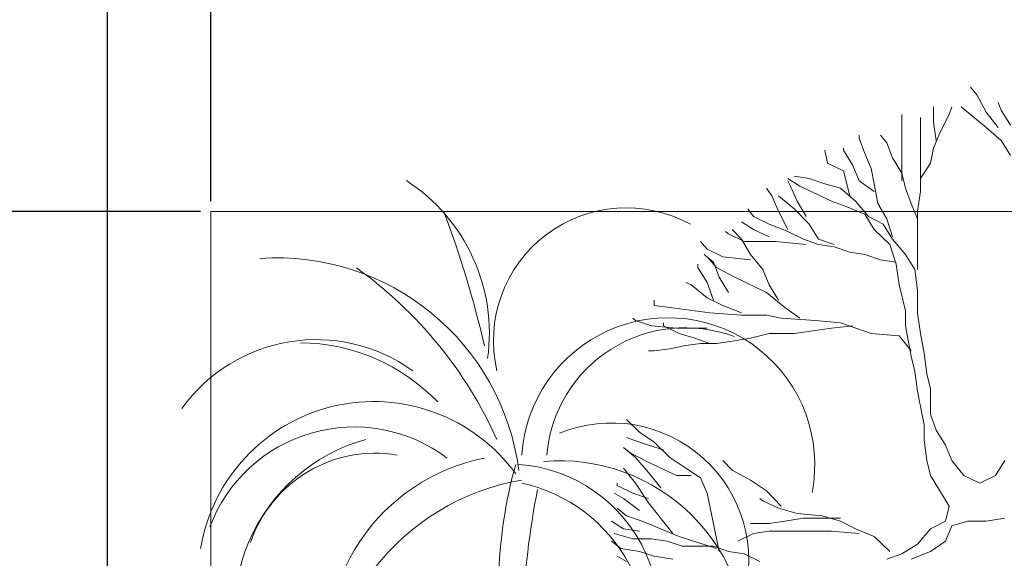
# Model space of a CAD drawing. Units: millimetres. Extents: x 595116 to 630915, y 909473 to 920225.
# Tile 51 of 134: x 629500 to 629559, y 919281 to 919314. Entities that reach past the tile are written whole.
import ezdxf

# ---------------------------------------------------------------- set-up
doc = ezdxf.new("R2010")
doc.units = ezdxf.units.MM
doc.layers.add('Dimension', color=3, linetype='Continuous', lineweight=18)
doc.layers.add('L-PLNT', color=85, linetype='Continuous', lineweight=13)
doc.styles.get("Standard").update_dxf_attribs({"font": 'arial.ttf'})
doc.dimstyles.new('ISO-25', dxfattribs={"dimtxt": 9, "dimasz": 6, "dimexe": 1.25, "dimexo": 0.625, "dimtad": 1, "dimlunit": 4, "dimtxsty": 'Standard', "dimcen": 2.5, "dimadec": 0, "dimazin": 0, "dimtfac": 1, "dimtmove": 0, "dimatfit": 3, "dimfxl": 1, "dimarcsym": 0})

# ---------------------------------------------------------------- blocks, each defined once
blk = doc.blocks.new('tree')
for centre, radius, start, end in [((629595.141, 919296.95), 5.184, 352.032, 57.0714), ((629569.835, 919289.496), 31.168, 13.149, 20.5076), ((629604.232, 919296.737), 3.791, 61.1347, 193.108), ((629594.259, 919292.132), 6.965, 7.4001, 94.0059), ((629589.446, 919288.922), 12.167, 24.2477, 54.3726), ((629605.429, 919293.205), 4.185, 348.9977, 176.315), ((629605.915, 919293.144), 3.963, 69.3845, 175.231), ((629595.377, 919292.044), 4.722, 54.2484, 144.2167), ((629594.88, 919291.171), 5.506, 43.8672, 89.4805), ((629597.025, 919289.989), 5.01, 36.0581, 170.6542), ((629596.464, 919289.874), 4.4, 52.9074, 159.3471), ((629603.809, 919290.469), 3.92, 343.886, 112.2662), ((629598.153, 919288.998), 5.103, 105.3576, 208.8973), ((629597.068, 919289.758), 3.768, 80.4816, 161.0664), ((629601.247, 919287.941), 5.545, 101.0419, 191.8692), ((629614.329, 919289.554), 13.748, 164.5925, 192.323), ((629600.849, 919288.894), 4.324, 322.5461, 85.805), ((629602.329, 919287.957), 5.355, 355.2141, 94.8217), ((629602.391, 919286.088), 6.769, 99.681, 184.5451), ((629626.813, 919287.645), 25.579, 169.0753, 185.2889), ((629600.275, 919288.191), 4.585, 338.7925, 77.6921)]:
    blk.add_arc(centre, radius, start, end)
blk = doc.blocks.new('A$C143125F4')
for p, q in [((2.1554, 4.9368), (2.1171, 4.9816)), ((2.2101, 4.8338), (2.1554, 4.9368)), ((2.2976, 4.8472), (2.2812, 4.892)), ((1.7123, 4.4306), (1.7123, 4.8203)), ((1.8983, 4.7755), (1.8983, 4.8651)), ((1.9366, 4.7128), (1.9913, 4.8203)), ((1.9913, 4.8203), (2.0077, 4.8651)), ((2.2101, 4.7442), (2.0624, 4.8651)), ((2.2812, 4.7442), (2.2101, 4.8338)), ((2.3523, 4.7576), (2.2976, 4.8472)), ((1.8217, 4.3679), (1.8217, 4.8024)), ((1.9147, 4.668), (1.8983, 4.7755)), ((1.8983, 4.6232), (1.9366, 4.7128)), ((2.2976, 4.668), (2.2101, 4.7442)), ((1.4606, 4.6814), (1.4606, 4.6994)), ((1.4935, 4.5919), (1.4606, 4.6814)), ((1.6247, 4.6546), (1.5865, 4.6994)), ((1.6576, 4.565), (1.6247, 4.6546)), ((2.3523, 4.5784), (2.2976, 4.668)), ((1.2746, 4.5336), (1.2582, 4.6098)), ((1.3676, 4.6098), (1.3676, 4.6232)), ((1.4223, 4.5202), (1.3676, 4.6098)), ((1.5317, 4.5023), (1.4935, 4.5919)), ((1.8819, 4.5336), (1.8983, 4.6232)), ((1.3676, 4.4888), (1.2746, 4.5336)), ((1.7123, 4.4754), (1.6576, 4.565)), ((1.8217, 4.444), (1.8819, 4.5336)), ((1.4059, 4.341), (1.3676, 4.4888)), ((1.4606, 4.4306), (1.4223, 4.5202)), ((1.5482, 4.4127), (1.5317, 4.5023)), ((1.7342, 4.3858), (1.7123, 4.4754)), ((1.1105, 4.3992), (1.0394, 4.444)), ((1.0558, 4.3992), (1.0394, 4.4306)), ((1.0777, 4.4575), (1.1652, 4.444)), ((1.1652, 4.444), (1.2582, 4.4127)), ((1.5482, 4.3679), (1.4606, 4.4306)), ((0.9464, 4.341), (0.9136, 4.3858)), ((1.0941, 4.3096), (1.0558, 4.3992)), ((1.2965, 4.3096), (1.1105, 4.3992)), ((1.2582, 4.4127), (1.3512, 4.3858)), ((1.3512, 4.3858), (1.4387, 4.3096)), ((1.57, 4.2962), (1.5482, 4.4127)), ((1.767, 4.2962), (1.7342, 4.3858)), ((1.8053, 4.2514), (1.8217, 4.3679)), ((0.9847, 4.2514), (0.9464, 4.341)), ((1.0777, 4.2648), (0.9847, 4.341)), ((1.1488, 4.22), (1.0941, 4.3096)), ((1.384, 4.2783), (1.2965, 4.3096)), ((1.4387, 4.3096), (1.5153, 4.22)), ((0.837, 4.22), (0.8042, 4.2648)), ((1.0394, 4.1439), (0.9847, 4.2514)), ((1.1652, 4.1752), (1.0777, 4.2648)), ((1.4935, 4.2335), (1.384, 4.2783)), ((1.6247, 4.2066), (1.57, 4.2962)), ((1.8053, 4.2066), (1.767, 4.2962)), ((1.8053, 3.9064), (1.8053, 4.2514)), ((0.837, 4.1439), (0.7659, 4.1887)), ((0.93, 4.1752), (0.837, 4.22)), ((1.5482, 4.1439), (1.4935, 4.2335)), ((1.5153, 4.22), (1.6029, 4.1752)), ((1.6576, 4.0991), (1.6247, 4.2066)), ((0.6893, 4.117), (0.6729, 4.1304)), ((0.7659, 4.0856), (0.7112, 4.1439)), ((0.93, 4.0991), (0.837, 4.1439)), ((1.0394, 4.1304), (0.93, 4.1752)), ((1.1324, 4.0856), (1.0394, 4.1304)), ((1.2199, 4.0856), (1.1652, 4.1752)), ((1.6412, 4.0543), (1.5482, 4.1439)), ((1.6029, 4.1752), (1.6576, 4.0856)), ((0.5635, 4.0274), (0.5252, 4.0722)), ((0.7823, 4.0722), (0.6893, 4.117)), ((0.8206, 3.996), (0.7659, 4.0856)), ((0.9683, 4.0722), (0.7823, 4.0722)), ((1.1488, 4.0543), (0.9683, 4.0722)), ((1.2199, 4.0543), (1.1324, 4.0856)), ((1.3129, 4.0543), (1.2199, 4.0856)), ((1.6576, 4.0856), (1.7342, 3.996)), ((0.6565, 3.9826), (0.5635, 4.0274)), ((1.3129, 4.0408), (1.2199, 4.0543)), ((1.4059, 4.0095), (1.3129, 4.0408)), ((1.4935, 3.996), (1.4059, 4.0095)), ((1.6795, 3.9378), (1.6412, 4.0543)), ((0.6018, 3.9512), (0.5471, 3.996)), ((0.6182, 3.9199), (0.5635, 3.9826)), ((0.6346, 3.8616), (0.6018, 3.9512)), ((0.8206, 3.9647), (0.6565, 3.9826)), ((0.8917, 3.9064), (0.8206, 3.996)), ((1.5865, 3.9647), (1.4935, 3.996)), ((1.6795, 3.9512), (1.5865, 3.9647)), ((1.7342, 3.996), (1.7889, 3.9064)), ((0.5088, 3.9199), (0.5088, 3.9378)), ((0.5635, 3.8303), (0.5088, 3.9199)), ((0.7276, 3.8616), (0.6182, 3.9199)), ((0.93, 3.8168), (0.8917, 3.9064)), ((1.6959, 3.8168), (1.6795, 3.9378)), ((1.7889, 3.9064), (1.8053, 3.7855)), ((0.6893, 3.772), (0.6346, 3.8616)), ((0.9136, 3.772), (0.7276, 3.8616)), ((0.4705, 3.8168), (0.4376, 3.8303)), ((0.5635, 3.7407), (0.4705, 3.8168)), ((0.6018, 3.7272), (0.5635, 3.8303)), ((0.9847, 3.7272), (0.93, 3.8168)), ((1.7342, 3.6645), (1.6959, 3.8168)), ((1.8053, 3.7855), (1.8053, 3.6511)), ((0.2516, 3.6959), (0.2516, 3.7272)), ((0.6565, 3.6959), (0.5635, 3.7407)), ((1.023, 3.6824), (0.9136, 3.772)), ((0.3446, 3.6824), (0.2516, 3.6959)), ((0.4923, 3.6645), (0.3446, 3.6824)), ((0.5799, 3.6511), (0.4923, 3.6645)), ((0.7659, 3.6511), (0.6565, 3.6959)), ((1.1105, 3.6197), (1.023, 3.6824)), ((1.7342, 3.5749), (1.7342, 3.6645)), ((0.1422, 3.6063), (0.1258, 3.6197)), ((0.2352, 3.5749), (0.1422, 3.6063)), ((0.7659, 3.6376), (0.5799, 3.6511)), ((0.9136, 3.6376), (0.7659, 3.6376)), ((1.0011, 3.6197), (0.9136, 3.6376)), ((1.2035, 3.6063), (1.0011, 3.6197)), ((1.3512, 3.5928), (1.2035, 3.6063)), ((1.8053, 3.6511), (1.8217, 3.5301)), ((0.3829, 3.5615), (0.2352, 3.5749)), ((0.3063, 3.5749), (0.3063, 3.5928)), ((0.3993, 3.5301), (0.3063, 3.5749)), ((0.5635, 3.5615), (0.3829, 3.5615)), ((1.2965, 3.5615), (1.0777, 3.5301)), ((1.4223, 3.5749), (1.2965, 3.5615)), ((1.5317, 3.5301), (1.3512, 3.5928)), ((1.767, 3.3957), (1.7342, 3.5749)), ((0.4923, 3.5032), (0.3993, 3.5301)), ((0.5799, 3.4719), (0.4923, 3.5032)), ((0.7112, 3.4853), (0.6182, 3.4719)), ((0.8206, 3.5032), (0.7112, 3.4853)), ((0.93, 3.5301), (0.8206, 3.5032)), ((1.0777, 3.5301), (0.93, 3.5301)), ((1.6959, 3.5167), (1.5317, 3.5301)), ((1.767, 3.4271), (1.6959, 3.5167)), ((1.8217, 3.5301), (1.8436, 3.4136)), ((0.2516, 3.4271), (0.2188, 3.4271)), ((0.3446, 3.4405), (0.2516, 3.4271)), ((0.4376, 3.4584), (0.3446, 3.4405)), ((0.5252, 3.4719), (0.4376, 3.4584)), ((0.6182, 3.4719), (0.5252, 3.4719)), ((1.7889, 3.3061), (1.767, 3.3957)), ((1.8436, 3.4136), (1.86, 3.2927)), ((1.8053, 3.1897), (1.7889, 3.3061)), ((1.86, 3.2927), (1.8819, 3.2031)), ((1.8819, 3.2031), (1.8819, 3.0553)), ((1.8217, 3.1001), (1.8053, 3.1897)), ((1.8436, 2.9925), (1.8217, 3.1001)), ((0.1641, 2.9477), (0.0875, 3.0239)), ((1.8819, 3.0553), (1.9147, 2.9612)), ((1.8436, 2.9029), (1.8436, 2.9925)), ((0.1258, 2.9029), (0.0875, 2.9164)), ((0.2516, 2.8895), (0.1641, 2.9477)), ((1.9147, 2.9612), (1.9694, 2.8716)), ((0.1422, 2.7999), (0.0711, 2.8581)), ((0.1094, 2.8268), (0.0711, 2.8581)), ((0.2188, 2.8716), (0.1258, 2.9029)), ((0.3063, 2.8447), (0.2188, 2.8716)), ((0.3446, 2.7999), (0.2516, 2.8895)), ((1.86, 2.782), (1.8436, 2.9029)), ((1.9694, 2.8716), (2.0077, 2.782)), ((0.1969, 2.782), (0.1094, 2.8268)), ((0.2188, 2.7103), (0.1422, 2.7999)), ((0.4376, 2.7372), (0.3446, 2.7999)), ((0.1422, 2.6476), (0.0711, 2.7372)), ((0.3829, 2.6924), (0.1969, 2.782)), ((0.5252, 2.679), (0.4376, 2.7372)), ((0.7112, 2.7238), (0.6565, 2.782)), ((1.8819, 2.6924), (1.86, 2.782)), ((2.0077, 2.782), (2.0788, 2.6924)), ((2.2648, 2.6924), (2.3195, 2.782)), ((0.2899, 2.6207), (0.2188, 2.7103)), ((0.4705, 2.6924), (0.3829, 2.6924)), ((0.5635, 2.5894), (0.5252, 2.679)), ((0.8206, 2.6655), (0.7112, 2.7238)), ((1.9913, 2.5132), (1.8819, 2.6924)), ((2.0788, 2.6924), (2.1718, 2.6476)), ((2.1718, 2.6476), (2.2648, 2.6924)), ((0.0328, 2.6342), (0.0328, 2.6476)), ((0.1258, 2.5894), (0.0328, 2.6342)), ((0.2188, 2.5311), (0.1422, 2.6476)), ((0.9136, 2.6028), (0.8206, 2.6655)), ((0.0711, 2.558), (0.0164, 2.5894)), ((0.1641, 2.4863), (0.0711, 2.558)), ((0.2188, 2.558), (0.1258, 2.5894)), ((0.6346, 2.2444), (0.5635, 2.5894)), ((0.8917, 2.5446), (0.8753, 2.558)), ((1.0011, 2.5132), (0.9136, 2.6028)), ((0.0875, 2.455), (0.0328, 2.4998)), ((0.3611, 2.3519), (0.2188, 2.5311)), ((0.9847, 2.4998), (0.8917, 2.5446)), ((1.0941, 2.4684), (0.9847, 2.4998)), ((1.9694, 2.4236), (1.9913, 2.5132)), ((0.1805, 2.4236), (0.0875, 2.455)), ((1.1324, 2.4415), (1.023, 2.4236)), ((1.2418, 2.455), (1.0941, 2.4684)), ((1.3512, 2.4415), (1.1324, 2.4415)), ((1.3512, 2.4236), (1.2418, 2.455)), ((2.3195, 2.4415), (2.2101, 2.4236)), ((0.0711, 2.3788), (0, 2.4236)), ((0.3993, 2.334), (0.1805, 2.4236)), ((0.93, 2.4102), (0.8206, 2.4102)), ((1.023, 2.4236), (0.93, 2.4102)), ((1.4387, 2.3788), (1.3512, 2.4236)), ((1.8819, 2.3788), (1.9694, 2.4236)), ((2.0077, 2.3967), (1.9694, 2.3071)), ((2.1007, 2.4236), (2.0077, 2.3967)), ((2.2101, 2.4236), (2.1007, 2.4236)), ((0.0164, 2.3519), (0.1258, 2.3206)), ((0.1641, 2.3654), (0.0711, 2.3788)), ((0.6182, 2.2623), (0.3993, 2.334)), ((0.837, 2.3519), (0.744, 2.3071)), ((0.93, 2.3654), (0.837, 2.3519)), ((1.2965, 2.3654), (0.93, 2.3654)), ((1.4606, 2.3519), (1.2965, 2.3654)), ((1.5482, 2.334), (1.4387, 2.3788)), ((1.6412, 2.2444), (1.5482, 2.334)), ((1.8053, 2.2892), (1.8819, 2.3788)), ((0.0547, 2.2623), (0, 2.3071)), ((0.1258, 2.3206), (0.2352, 2.3206)), ((0.2352, 2.3206), (0.3282, 2.3071)), ((0.3282, 2.3071), (0.4158, 2.2758)), ((0.4158, 2.2758), (0.6018, 2.2758)), ((0.6018, 2.2758), (0.6893, 2.2444)), ((1.7123, 2.231), (1.8053, 2.2892)), ((1.9694, 2.3071), (1.8819, 2.2444)), ((0.0875, 2.1862), (0.0328, 2.2175)), ((0.1641, 2.2444), (0.0547, 2.2623)), ((0.2516, 2.2175), (0.1641, 2.2444)), ((0.3611, 2.1996), (0.2516, 2.2175)), ((0.6893, 2.2444), (0.7823, 2.231)), ((0.7823, 2.231), (0.8753, 2.1862)), ((1.6247, 2.1996), (1.7123, 2.231)), ((1.8819, 2.2444), (1.767, 2.1996))]:
    blk.add_line(p, q)
blk = doc.blocks.new('*D215')
at = {"layer": 'Defpoints', "color": 0, "transparency": 16777216}
for p in [(629316.041, 919411.828), (629505.041, 919411.828), (629505.041, 918832.378)]:
    blk.add_point(p, dxfattribs=at)
at = {"layer": 'Dimension', "color": 0, "lineweight": -2, "transparency": 16777216}
for p, q in [((629316.041, 919411.203), (629316.041, 918831.128)), ((629505.041, 919411.203), (629505.041, 918831.128)), ((629322.041, 918832.378), (629499.041, 918832.378))]:
    blk.add_line(p, q, dxfattribs=at)
at = {"layer": 'Dimension', "color": 0, "transparency": 16777216}
for points in [[(629322.041, 918833.378), (629322.041, 918831.378), (629316.041, 918832.378)], [(629499.041, 918833.378), (629499.041, 918831.378), (629505.041, 918832.378)]]:
    blk.add_solid(points, dxfattribs=at)
at = {"layer": 'Dimension', "color": 0, "transparency": 16777216, "insert": (629410.541, 918837.598), "char_height": 9, "attachment_point": 5}
blk.add_mtext('15\'-9"', dxfattribs=at)
blk = doc.blocks.new('*D216')
at = {"layer": 'Defpoints', "color": 0, "transparency": 16777216}
for p in [(629505.041, 919411.828), (629743.541, 919411.928), (629743.541, 918832.378)]:
    blk.add_point(p, dxfattribs=at)
at = {"layer": 'Dimension', "color": 0, "lineweight": -2, "transparency": 16777216}
for p, q in [((629505.041, 919411.203), (629505.041, 918831.128)), ((629743.541, 919411.303), (629743.541, 918831.128)), ((629511.041, 918832.378), (629737.541, 918832.378))]:
    blk.add_line(p, q, dxfattribs=at)
at = {"layer": 'Dimension', "color": 0, "transparency": 16777216}
for points in [[(629511.041, 918833.378), (629511.041, 918831.378), (629505.041, 918832.378)], [(629737.541, 918833.378), (629737.541, 918831.378), (629743.541, 918832.378)]]:
    blk.add_solid(points, dxfattribs=at)
at = {"layer": 'Dimension', "color": 0, "transparency": 16777216, "insert": (629624.291, 918837.656), "char_height": 9, "attachment_point": 5}
blk.add_mtext('19\'-10 1/2"', dxfattribs=at)
blk = doc.blocks.new('*D220')
at = {"layer": 'Defpoints', "color": 0, "transparency": 16777216}
for p in [(629824.951, 920160.756), (629511.274, 919302.009), (629824.951, 919302.009)]:
    blk.add_point(p, dxfattribs=at)
at = {"layer": 'Dimension', "color": 0, "lineweight": -2, "transparency": 16777216}
for p, q in [((629511.274, 919302.634), (629511.274, 920162.006)), ((629824.951, 919302.634), (629824.951, 920162.006)), ((629517.274, 920160.756), (629818.951, 920160.756))]:
    blk.add_line(p, q, dxfattribs=at)
at = {"layer": 'Dimension', "color": 0, "transparency": 16777216}
for points in [[(629517.274, 920161.756), (629517.274, 920159.756), (629511.274, 920160.756)], [(629818.951, 920161.756), (629818.951, 920159.756), (629824.951, 920160.756)]]:
    blk.add_solid(points, dxfattribs=at)
at = {"layer": 'Dimension', "color": 0, "transparency": 16777216, "insert": (629668.113, 920166.035), "char_height": 9, "attachment_point": 5}
blk.add_mtext('26\'-1 1/2"', dxfattribs=at)
blk = doc.blocks.new('*D221')
at = {"layer": 'Defpoints', "color": 0, "transparency": 16777216}
for p in [(629511.274, 919302.009), (629155.382, 919160.917), (629511.274, 919160.917)]:
    blk.add_point(p, dxfattribs=at)
at = {"layer": 'Dimension', "color": 0, "lineweight": -2, "transparency": 16777216}
for p, q in [((629510.649, 919302.009), (629154.132, 919302.009)), ((629155.382, 919296.009), (629155.382, 919166.917)), ((629510.649, 919160.917), (629154.132, 919160.917))]:
    blk.add_line(p, q, dxfattribs=at)
at = {"layer": 'Dimension', "color": 0, "transparency": 16777216}
for points in [[(629154.382, 919296.009), (629156.382, 919296.009), (629155.382, 919302.009)], [(629154.382, 919166.917), (629156.382, 919166.917), (629155.382, 919160.917)]]:
    blk.add_solid(points, dxfattribs=at)
at = {"layer": 'Dimension', "color": 0, "transparency": 16777216, "insert": (629150.162, 919231.463), "char_height": 9, "attachment_point": 5, "rotation": 90}
blk.add_mtext('11\'-9"', dxfattribs=at)

msp = doc.modelspace()

# ---------------------------------------------------------------- linework, layer by layer
at = {"layer": 'L-PLNT'}
for p, q in [((629824.951, 919302.009), (629511.274, 919302.009)), ((629511.274, 919302.009), (629511.274, 919160.917))]:
    msp.add_line(p, q, dxfattribs=at)

# ---------------------------------------------------------------- block references
for name, p, xscale, yscale, zscale in [('A$C143125F4', (629535.386, 919258.662), 10.20167662382051, 10.20167662382051, 10.20167662382051), ('tree', (-697473.9, -1018297.752), 2.107689410566463, 2.107689410566463, 2.107689410566463)]:
    msp.add_blockref(name, p, dxfattribs=dict(at, xscale=xscale, yscale=yscale, zscale=zscale))

# ---------------------------------------------------------------- dimensions: what is measured, and where the dimension line sits
at = {"layer": 'Dimension'}
for base, p1, p2, picture, middle in [((629824.951, 920160.756), (629511.274, 919302.009), (629824.951, 919302.009), '*D220', (629668.113, 920166.035)), ((629505.041, 918832.378), (629316.041, 919411.828), (629505.041, 919411.828), '*D215', (629410.541, 918837.598)), ((629743.541, 918832.378), (629505.041, 919411.828), (629743.541, 919411.928), '*D216', (629624.291, 918837.656))]:
    dim = msp.add_linear_dim(base=base, p1=p1, p2=p2, dimstyle='ISO-25', override={"dimdec": 1, "dimlfac": 1, "dimrnd": 0, "dimzin": 1, "dimdsep": 46, "dimlunit": 4, "dimfrac": 2}, dxfattribs=at)
    dim.commit()
    dim.dimension.update_dxf_attribs({"geometry": picture, "text_midpoint": middle})
dim = msp.add_linear_dim(base=(629155.382, 919160.917), p1=(629511.274, 919302.009), p2=(629511.274, 919160.917), angle=90, dimstyle='ISO-25', override={"dimdec": 1, "dimlfac": 1, "dimrnd": 0, "dimzin": 1, "dimdsep": 46, "dimlunit": 4, "dimfrac": 2}, dxfattribs=at)
dim.commit()
dim.dimension.update_dxf_attribs({"geometry": '*D221', "text_midpoint": (629150.162, 919231.463)})

doc.saveas('drawing.dxf')
